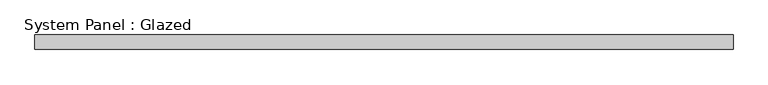
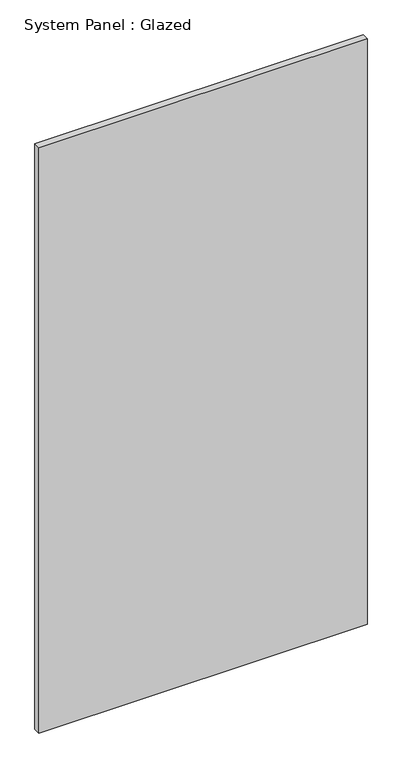
"""IFC4 building model written with IfcOpenShell, lengths in millimetres: plate geometry, System Panel : Glazed."""

from ifc_helpers import new_model, si_unit, origin, origin_with_axes, place, context, project, spatial, polyline, outline, extrude, source, transform, mapped, element, save


def system_panel_glazed_6119edd6(model_context):
    return source(origin(), model_context, "Body", "SweptSolid", [
        extrude(outline(polyline([(612.7750001, 19.05), (-612.7750001, 19.05), (-612.7750001, 44.45), (612.7750001, 44.45), (612.7750001, 19.05)])), origin_with_axes(), (0.0, 0.0, 1.0), 2311.4),
    ])


if __name__ == "__main__":
    model = new_model("IFC4")
    model_context = context("Model", 3, world=origin())
    ifc_project = project(units=[si_unit("LENGTHUNIT", "METRE", prefix="MILLI")], contexts=[model_context])
    site = spatial("IfcSite", under=ifc_project)
    building = spatial("IfcBuilding", under=site)
    placement = place(None, origin())
    system_panel_glazed_shape = system_panel_glazed_6119edd6(model_context)
    element("IfcPlate", 1, ObjectType="System Panel : Glazed", at=placement, inside=building, context=model_context, shape_type="MappedRepresentation", body=[
        mapped(system_panel_glazed_shape, transform((0.0, 0.0, 0.0), x_axis=(1.0, 0.0, 0.0), y_axis=(0.0, 1.0, 0.0), z_axis=(0.0, 0.0, 1.0))),
    ])
    save(model, "model.ifc")

# Revit data of these elements
# Type "System Panel : Glazed"
#   Construction Type Id = "GSP4R"
#   Analytic Construction = "1/8 in Pilkington single glazing"
#   Visual Light Transmittance = 0.9
#   Solar Heat Gain Coefficient = 0.86
#   Heat Transfer Coefficient (U) = 1.18115 BTU/(h·ft²·°F)
#   Define Thermal Properties by = 1
# Element 1 (IfcPlate, "System Panel : Glazed")
#   Materials on its faces: "Glass"
# Materials
#   "Glass": class "Glass", colour RGB 0 128 192, transparency 0.75, Description = "Soda Lime Glass", Cost = 0
